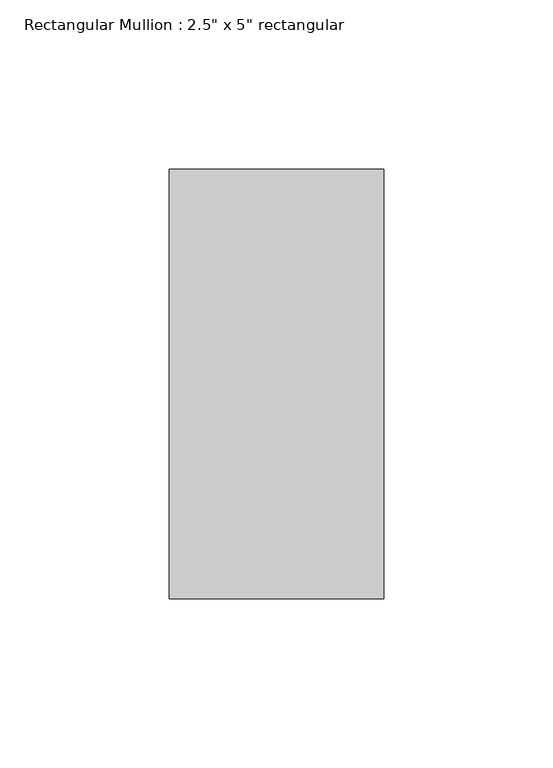
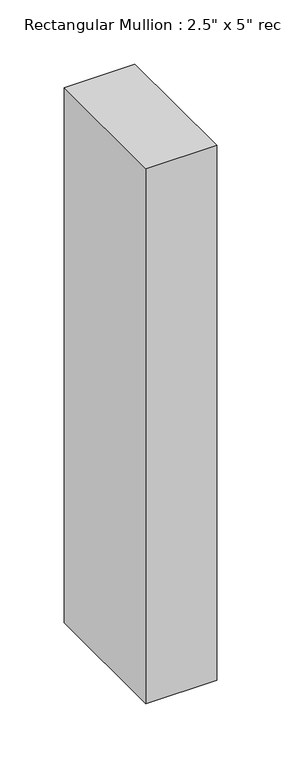
"""IFC4 building model written with IfcOpenShell, lengths in millimetres: member geometry."""

from ifc_helpers import new_model, si_unit, frame, origin, place, context, project, spatial, polyline, outline, extrude, source, transform, mapped, element, save


def member_90750a43(model_context):
    return source(origin(), model_context, "Body", "SweptSolid", [
        extrude(outline(polyline([(31.75, 63.5), (31.75, -63.5), (-31.75, -63.5), (-31.75, 63.5), (31.75, 63.5)])), frame((0.0, 0.0, -508.0), z_axis=(0.0, 0.0, 1.0), x_axis=(1.0, 0.0, 0.0)), (0.0, 0.0, 1.0), 508.0),
    ])


if __name__ == "__main__":
    model = new_model("IFC4")
    model_context = context("Model", 3, world=origin())
    ifc_project = project(units=[si_unit("LENGTHUNIT", "METRE", prefix="MILLI")], contexts=[model_context])
    site = spatial("IfcSite", under=ifc_project)
    building = spatial("IfcBuilding", under=site)
    placement = place(None, origin())
    member_shape = member_90750a43(model_context)
    element("IfcMember", 1, ObjectType="Rectangular Mullion : 2.5\" x 5\" rectangular", at=placement, inside=building, context=model_context, shape_type="MappedRepresentation", body=[
        mapped(member_shape, transform((0.0, 0.0, 0.0), x_axis=(1.0, 0.0, 0.0), y_axis=(0.0, 1.0, 0.0), z_axis=(0.0, 0.0, 1.0))),
    ])
    save(model, "model.ifc")

# Revit data of these elements
# Type "Rectangular Mullion : 2.5\" x 5\" rectangular"
#   built-in parameter 1007304 = 0.416667 (stored number, unit not read)
#   built-in parameter 1007301 = 0.104167 (stored number, unit not read)
#   built-in parameter 1007300 = 0.104167 (stored number, unit not read)
# Element 1 (IfcMember, "Rectangular Mullion : 2.5\" x 5\" rectangular")
#   Materials on its faces: "Rectangle 1 sq"
# Materials
#   "Rectangle 1 sq": class "Generic", colour RGB 120 120 120, transparency 0, Cost = 0
